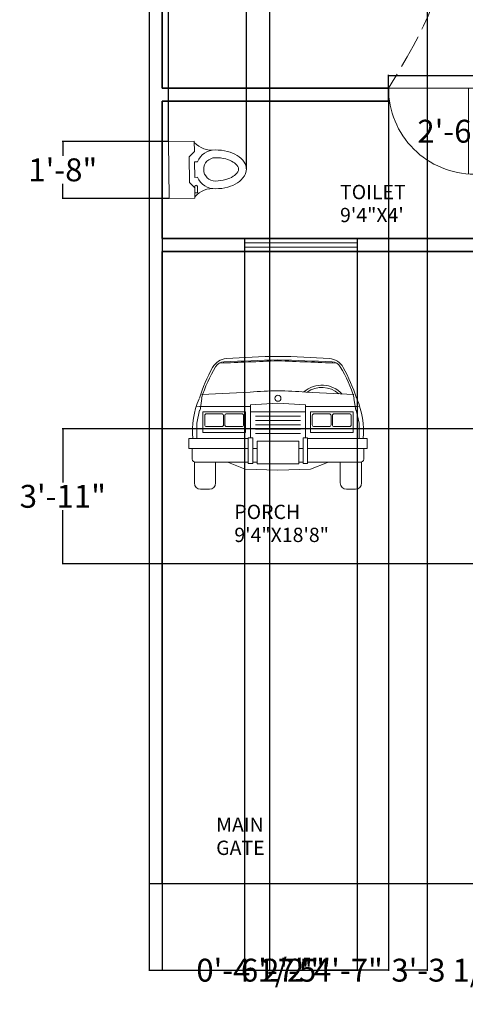
# Model space of a CAD drawing. Units: inches. Extents: x -26 to 385, y 12 to 697.
# Tile 1 of 13: x -20 to 136, y 12 to 356. Entities that reach past the tile are written whole.
import ezdxf

# ---------------------------------------------------------------- set-up
doc = ezdxf.new("R2010")
doc.units = ezdxf.units.IN
doc.header["$MEASUREMENT"] = 0
doc.linetypes.add('ACAD_ISO02W100', pattern=[15, 12, -3])
for name, color, linetype, lineweight in [('A-ANNO-DIMS', 4, 'Continuous', 18), ('A-ANNO-TEXT', 7, 'Continuous', 18), ('A-AREA-IDEN', 4, 'Continuous', 18), ('A-DOOR', 30, 'Continuous', 20), ('A-EQPM-VEHI', 7, 'Continuous', 15), ('A-FLOR-FIXT', 7, 'Continuous', 18), ('A-FLOR-OVHD', 3, 'ACAD_ISO02W100', 13), ('A-GLAZ', 5, 'Continuous', 18), ('A-WALL', 40, 'Continuous', 35), ('C-PROP', 40, 'Continuous', 25)]:
    doc.layers.add(name, color=color, linetype=linetype, lineweight=lineweight)
doc.styles.get("Standard").update_dxf_attribs({"font": 'italic8.shx'})
doc.dimstyles.get("Standard").update_dxf_attribs({"dimtxt": 8, "dimasz": 0.18, "dimexe": 0.18, "dimexo": 0.0625, "dimgap": 0.09, "dimtad": 0, "dimtih": 1, "dimtoh": 1, "dimdec": 4, "dimzin": 0, "dimdsep": 46, "dimlunit": 3, "dimtxsty": 'Standard', "dimcen": 0.09, "dimclrd": 2, "dimclre": 3, "dimclrt": 6, "dimadec": 0, "dimazin": 0, "dimtfac": 1, "dimtdec": 4, "dimtofl": 0, "dimtmove": 0, "dimatfit": 3, "dimfxl": 1, "dimtolj": 1, "dimtzin": 0, "dimarcsym": 0})

# ---------------------------------------------------------------- blocks, each defined once
blk = doc.blocks.new('DOOR-SWING-30IN')
for p, q in [((0, -30), (0, 0)), ((0, 0), (30, 0)), ((0, -2), (30, -2))]:
    blk.add_line(p, q)
blk.add_arc((0, 0), 30, 270, 0)
blk = doc.blocks.new('*D17')
at = {"layer": 'A-ANNO-DIMS', "color": 3, "lineweight": -2, "transparency": 16777216}
for p, q in [((108.79, 332.44), (108.79, 337.06)), ((138.79, 332.44), (138.79, 337.06))]:
    blk.add_line(p, q, dxfattribs=at)
at = {"layer": 'A-ANNO-DIMS', "color": 2, "lineweight": -2, "transparency": 16777216}
for p, q in [((108.97, 336.88), (138.61, 336.88)), ((138.79, 336.88), (138.97, 336.88))]:
    blk.add_line(p, q, dxfattribs=at)
at = {"layer": 'A-ANNO-DIMS', "color": 2, "transparency": 16777216}
for points in [[(108.97, 336.91), (108.97, 336.85), (108.79, 336.88)], [(138.61, 336.91), (138.61, 336.85), (138.79, 336.88)]]:
    blk.add_solid(points, dxfattribs=at)
at = {"layer": 'Defpoints', "color": 0, "transparency": 16777216}
for p in [(138.79, 336.88), (108.79, 332.38), (138.79, 332.38)]:
    blk.add_point(p, dxfattribs=at)
at = {"layer": 'A-ANNO-DIMS', "color": 6, "transparency": 16777216, "insert": (196.21, 336.88), "char_height": 8, "attachment_point": 5}
blk.add_mtext('\\A1;DOOR 2\'-6" TYP.', dxfattribs=at)
blk = doc.blocks.new('*D18')
at = {"layer": 'A-ANNO-DIMS', "color": 3, "lineweight": -2, "transparency": 16777216}
for p, q in [((138.86, 332.38), (143.47, 332.38)), ((138.86, 302.38), (143.47, 302.38))]:
    blk.add_line(p, q, dxfattribs=at)
at = {"layer": 'A-ANNO-DIMS', "color": 2, "lineweight": -2, "transparency": 16777216}
for p, q in [((143.29, 332.2), (143.29, 322.23)), ((143.29, 302.56), (143.29, 312.53))]:
    blk.add_line(p, q, dxfattribs=at)
at = {"layer": 'A-ANNO-DIMS', "color": 2, "transparency": 16777216}
for points in [[(143.26, 332.2), (143.32, 332.2), (143.29, 332.38)], [(143.26, 302.56), (143.32, 302.56), (143.29, 302.38)]]:
    blk.add_solid(points, dxfattribs=at)
at = {"layer": 'Defpoints', "color": 0, "transparency": 16777216}
for p in [(138.79, 332.38), (138.79, 302.38), (143.29, 302.38)]:
    blk.add_point(p, dxfattribs=at)
at = {"layer": 'A-ANNO-DIMS', "color": 6, "transparency": 16777216, "insert": (143.29, 317.38), "char_height": 8, "attachment_point": 5}
blk.add_mtext('\\A1;2\'-6" TYP.', dxfattribs=at)
blk = doc.blocks.new('*D29')
at = {"layer": 'A-ANNO-DIMS', "color": 3, "lineweight": -2, "transparency": 16777216}
for p, q in [((67.17, 549.17), (67.17, 23.95)), ((122.29, 549.17), (122.29, 23.95))]:
    blk.add_line(p, q, dxfattribs=at)
at = {"layer": 'A-ANNO-DIMS', "color": 2, "lineweight": -2, "transparency": 16777216}
for p, q in [((67.35, 24.13), (76.92, 24.13)), ((122.11, 24.13), (112.53, 24.13))]:
    blk.add_line(p, q, dxfattribs=at)
at = {"layer": 'A-ANNO-DIMS', "color": 2, "transparency": 16777216}
for points in [[(67.35, 24.16), (67.35, 24.1), (67.17, 24.13)], [(122.11, 24.16), (122.11, 24.1), (122.29, 24.13)]]:
    blk.add_solid(points, dxfattribs=at)
at = {"layer": 'Defpoints', "color": 0, "transparency": 16777216}
for p in [(67.17, 549.23), (122.29, 549.23), (122.29, 24.13)]:
    blk.add_point(p, dxfattribs=at)
at = {"layer": 'A-ANNO-DIMS', "color": 6, "transparency": 16777216, "insert": (94.73, 24.13), "char_height": 8, "attachment_point": 5}
blk.add_mtext('\\A1;4\'-7"', dxfattribs=at)
blk = doc.blocks.new('*D32')
at = {"layer": 'A-ANNO-DIMS', "color": 3, "lineweight": -2, "transparency": 16777216}
for p, q in [((239.83, 213.39), (-5.3, 213.39)), ((239.83, 166.14), (-5.3, 166.14))]:
    blk.add_line(p, q, dxfattribs=at)
at = {"layer": 'A-ANNO-DIMS', "color": 2, "lineweight": -2, "transparency": 16777216}
for p, q in [((-5.12, 213.21), (-5.12, 194.62)), ((-5.12, 166.32), (-5.12, 184.91))]:
    blk.add_line(p, q, dxfattribs=at)
at = {"layer": 'A-ANNO-DIMS', "color": 2, "transparency": 16777216}
for points in [[(-5.15, 213.21), (-5.09, 213.21), (-5.12, 213.39)], [(-5.15, 166.32), (-5.09, 166.32), (-5.12, 166.14)]]:
    blk.add_solid(points, dxfattribs=at)
at = {"layer": 'Defpoints', "color": 0, "transparency": 16777216}
for p in [(-5.12, 213.39), (239.89, 213.39), (239.89, 166.14)]:
    blk.add_point(p, dxfattribs=at)
at = {"layer": 'A-ANNO-DIMS', "color": 6, "transparency": 16777216, "insert": (-5.12, 189.76), "char_height": 8, "attachment_point": 5}
blk.add_mtext('\\A1;3\'-11"', dxfattribs=at)
blk = doc.blocks.new('*D33')
at = {"layer": 'A-ANNO-DIMS', "color": 3, "lineweight": -2, "transparency": 16777216}
for p, q in [((58.47, 279.82), (58.47, 23.95)), ((97.85, 279.82), (97.85, 23.95))]:
    blk.add_line(p, q, dxfattribs=at)
at = {"layer": 'A-ANNO-DIMS', "color": 2, "lineweight": -2, "transparency": 16777216}
for p, q in [((58.65, 24.13), (97.67, 24.13)), ((97.85, 24.13), (98.03, 24.13))]:
    blk.add_line(p, q, dxfattribs=at)
at = {"layer": 'A-ANNO-DIMS', "color": 2, "transparency": 16777216}
for points in [[(58.65, 24.16), (58.65, 24.1), (58.47, 24.13)], [(97.67, 24.16), (97.67, 24.1), (97.85, 24.13)]]:
    blk.add_solid(points, dxfattribs=at)
at = {"layer": 'Defpoints', "color": 0, "transparency": 16777216}
for p in [(58.47, 279.88), (97.85, 279.88), (97.85, 24.13)]:
    blk.add_point(p, dxfattribs=at)
at = {"layer": 'A-ANNO-DIMS', "color": 6, "transparency": 16777216, "insert": (131.26, 24.13), "char_height": 8, "attachment_point": 5}
blk.add_mtext('\\A1;3\'-3 1/2"', dxfattribs=at)
blk = doc.blocks.new('*D34')
at = {"layer": 'A-ANNO-DIMS', "color": 3, "lineweight": -2, "transparency": 16777216}
for p, q in [((29.63, 279.82), (29.63, 23.95)), ((58.47, 279.82), (58.47, 23.95))]:
    blk.add_line(p, q, dxfattribs=at)
at = {"layer": 'A-ANNO-DIMS', "color": 2, "lineweight": -2, "transparency": 16777216}
for p, q in [((29.81, 24.13), (58.29, 24.13)), ((58.47, 24.13), (58.65, 24.13))]:
    blk.add_line(p, q, dxfattribs=at)
at = {"layer": 'A-ANNO-DIMS', "color": 2, "transparency": 16777216}
for points in [[(29.81, 24.16), (29.81, 24.1), (29.63, 24.13)], [(58.29, 24.16), (58.29, 24.1), (58.47, 24.13)]]:
    blk.add_solid(points, dxfattribs=at)
at = {"layer": 'Defpoints', "color": 0, "transparency": 16777216}
for p in [(29.63, 279.88), (58.47, 279.88), (58.47, 24.13)]:
    blk.add_point(p, dxfattribs=at)
at = {"layer": 'A-ANNO-DIMS', "color": 6, "transparency": 16777216, "insert": (76.64, 24.13), "char_height": 8, "attachment_point": 5}
blk.add_mtext('\\A1;2\'-5"', dxfattribs=at)
blk = doc.blocks.new('*D40')
at = {"layer": 'A-ANNO-DIMS', "color": 3, "lineweight": -2, "transparency": 16777216}
for p, q in [((31.75, 313.84), (-5.3, 313.84)), ((31.96, 293.92), (-5.3, 293.92))]:
    blk.add_line(p, q, dxfattribs=at)
at = {"layer": 'A-ANNO-DIMS', "color": 2, "lineweight": -2, "transparency": 16777216}
for p, q in [((-5.12, 313.66), (-5.12, 308.73)), ((-5.12, 294.1), (-5.12, 299.03))]:
    blk.add_line(p, q, dxfattribs=at)
at = {"layer": 'A-ANNO-DIMS', "color": 2, "transparency": 16777216}
for points in [[(-5.15, 313.66), (-5.09, 313.66), (-5.12, 313.84)], [(-5.15, 294.1), (-5.09, 294.1), (-5.12, 293.92)]]:
    blk.add_solid(points, dxfattribs=at)
at = {"layer": 'Defpoints', "color": 0, "transparency": 16777216}
for p in [(31.81, 313.84), (-5.12, 293.92), (32.02, 293.92)]:
    blk.add_point(p, dxfattribs=at)
at = {"layer": 'A-ANNO-DIMS', "color": 6, "transparency": 16777216, "insert": (-5.12, 303.88), "char_height": 8, "attachment_point": 5}
blk.add_mtext('\\A1;1\'-8"', dxfattribs=at)
blk = doc.blocks.new('*D41')
at = {"layer": 'A-ANNO-DIMS', "color": 3, "lineweight": -2, "transparency": 16777216}
for p, q in [((31.81, 313.9), (31.81, 684.81)), ((59.08, 304.23), (59.08, 684.81))]:
    blk.add_line(p, q, dxfattribs=at)
at = {"layer": 'A-ANNO-DIMS', "color": 2, "lineweight": -2, "transparency": 16777216}
for p, q in [((31.99, 684.63), (58.9, 684.63)), ((59.08, 684.63), (59.26, 684.63))]:
    blk.add_line(p, q, dxfattribs=at)
at = {"layer": 'A-ANNO-DIMS', "color": 2, "transparency": 16777216}
for points in [[(31.99, 684.66), (31.99, 684.6), (31.81, 684.63)], [(58.9, 684.66), (58.9, 684.6), (59.08, 684.63)]]:
    blk.add_solid(points, dxfattribs=at)
at = {"layer": 'Defpoints', "color": 0, "transparency": 16777216}
for p in [(59.08, 684.63), (31.81, 313.84), (59.08, 304.16)]:
    blk.add_point(p, dxfattribs=at)
at = {"layer": 'A-ANNO-DIMS', "color": 6, "transparency": 16777216, "insert": (92.49, 684.63), "char_height": 8, "attachment_point": 5}
blk.add_mtext('\\A1;2\'-3 1/2"', dxfattribs=at)
blk = doc.blocks.new('*D43')
at = {"layer": 'A-ANNO-DIMS', "color": 3, "lineweight": -2, "transparency": 16777216}
for p, q in [((25.13, 54.32), (25.13, 23.95)), ((29.63, 54.32), (29.63, 23.95))]:
    blk.add_line(p, q, dxfattribs=at)
at = {"layer": 'A-ANNO-DIMS', "color": 2, "lineweight": -2, "transparency": 16777216}
for p, q in [((25.31, 24.13), (29.45, 24.13)), ((29.63, 24.13), (29.81, 24.13))]:
    blk.add_line(p, q, dxfattribs=at)
at = {"layer": 'A-ANNO-DIMS', "color": 2, "transparency": 16777216}
for points in [[(25.31, 24.16), (25.31, 24.1), (25.13, 24.13)], [(29.45, 24.16), (29.45, 24.1), (29.63, 24.13)]]:
    blk.add_solid(points, dxfattribs=at)
at = {"layer": 'Defpoints', "color": 0, "transparency": 16777216}
for p in [(25.13, 54.38), (29.63, 54.38), (29.63, 24.13)]:
    blk.add_point(p, dxfattribs=at)
at = {"layer": 'A-ANNO-DIMS', "color": 6, "transparency": 16777216, "insert": (63.04, 24.13), "char_height": 8, "attachment_point": 5}
blk.add_mtext('\\A1;0\'-4 1/2"', dxfattribs=at)
blk = doc.blocks.new('*D47')
at = {"layer": 'A-ANNO-DIMS', "color": 3, "lineweight": -2, "transparency": 16777216}
for p, q in [((29.63, 327.82), (29.63, 23.95)), ((108.79, 327.82), (108.79, 23.95))]:
    blk.add_line(p, q, dxfattribs=at)
at = {"layer": 'A-ANNO-DIMS', "color": 2, "lineweight": -2, "transparency": 16777216}
for p, q in [((29.81, 24.13), (51.41, 24.13)), ((108.61, 24.13), (87.02, 24.13))]:
    blk.add_line(p, q, dxfattribs=at)
at = {"layer": 'A-ANNO-DIMS', "color": 2, "transparency": 16777216}
for points in [[(29.81, 24.16), (29.81, 24.1), (29.63, 24.13)], [(108.61, 24.16), (108.61, 24.1), (108.79, 24.13)]]:
    blk.add_solid(points, dxfattribs=at)
at = {"layer": 'Defpoints', "color": 0, "transparency": 16777216}
for p in [(29.63, 327.88), (108.79, 327.88), (108.79, 24.13)]:
    blk.add_point(p, dxfattribs=at)
at = {"layer": 'A-ANNO-DIMS', "color": 6, "transparency": 16777216, "insert": (69.21, 24.13), "char_height": 8, "attachment_point": 5}
blk.add_mtext('\\A1;6\'-7"', dxfattribs=at)

msp = doc.modelspace()

# ---------------------------------------------------------------- linework, layer by layer
at = {"layer": 'A-EQPM-VEHI'}
for p, q in [((43.52309, 223.97111), (42.85778, 219.9024)), ((60.39116, 226.18572), (43.52309, 225.29953)), ((79.84318, 226.18572), (96.71125, 225.29953)), ((96.71125, 223.97111), (97.37656, 219.9024)), ((43.01615, 221.16936), (41.74919, 221.32773)), ((42.70356, 221.18633), (60.51804, 221.18633)), ((60.51804, 221.74383), (70.11717, 222.33442)), ((60.51804, 210.2496), (60.51804, 221.74383)), ((79.7163, 221.74383), (70.11717, 222.33442)), ((79.7163, 210.2496), (79.7163, 221.74383)), ((97.53078, 221.18633), (79.7163, 221.18633)), ((97.21819, 221.16936), (98.48515, 221.32773)), ((42.71571, 219.85792), (41.74919, 215.30968)), ((43.83595, 212.09194), (43.83595, 219.28259)), ((43.83595, 219.28259), (58.7398, 219.28259)), ((44.49774, 217.94019), (44.49774, 214.79154)), ((50.4349, 218.59311), (45.15065, 218.59311)), ((51.08782, 217.94019), (51.08782, 214.79154)), ((51.53662, 217.94019), (51.53662, 214.79154)), ((57.47378, 218.59311), (52.18953, 218.59311)), ((58.12669, 214.79154), (58.12669, 217.94019)), ((58.7398, 219.28259), (58.7398, 212.09194)), ((60.51804, 219.28259), (79.7163, 219.28259)), ((78.01892, 217.75578), (62.21542, 217.75578)), ((96.39839, 219.28259), (81.49454, 219.28259)), ((81.49454, 219.28259), (81.49454, 212.09194)), ((82.10765, 214.79154), (82.10765, 217.94019)), ((82.76056, 218.59311), (88.04481, 218.59311)), ((88.69772, 217.94019), (88.69772, 214.79154)), ((89.14652, 217.94019), (89.14652, 214.79154)), ((89.79944, 218.59311), (95.08369, 218.59311)), ((95.7366, 217.94019), (95.7366, 214.79154)), ((96.39839, 212.09194), (96.39839, 219.28259)), ((97.51863, 219.85792), (98.48515, 215.30968)), ((41.74919, 215.30968), (41.74919, 209.94942)), ((45.15065, 214.13863), (50.4349, 214.13863)), ((52.18953, 214.13863), (57.47378, 214.13863)), ((78.01892, 216.25078), (62.21542, 216.25078)), ((78.01892, 214.74578), (62.21542, 214.74578)), ((88.04481, 214.13863), (82.76056, 214.13863)), ((95.08369, 214.13863), (89.79944, 214.13863)), ((98.48515, 215.30968), (98.48515, 209.94942)), ((38.90862, 209.94942), (59.74715, 209.94942)), ((38.90862, 206.4827), (38.90862, 209.94942)), ((58.7398, 212.09194), (43.83595, 212.09194)), ((59.74715, 210.2496), (59.74715, 201.2559)), ((61.28893, 210.2496), (59.74715, 210.2496)), ((61.28893, 201.2559), (61.28893, 210.2496)), ((78.01892, 213.24078), (62.21542, 213.24078)), ((78.01892, 211.73577), (62.21542, 211.73577)), ((78.94541, 210.2496), (80.48719, 210.2496)), ((78.94541, 201.2559), (78.94541, 210.2496)), ((80.48719, 210.2496), (80.48719, 201.2559)), ((101.32572, 209.94942), (80.48719, 209.94942)), ((81.49454, 212.09194), (96.39839, 212.09194)), ((101.32572, 206.4827), (101.32572, 209.94942)), ((62.8307, 201.17364), (62.8307, 209.05709)), ((62.8307, 209.05709), (77.40364, 209.05709)), ((77.40364, 201.17364), (77.40364, 209.05709)), ((38.90862, 206.4827), (59.74715, 206.4827)), ((40.07105, 202.71282), (40.07105, 206.49837)), ((61.28893, 206.4827), (62.8307, 206.4827)), ((77.40364, 206.4827), (78.94541, 206.4827)), ((101.32572, 206.4827), (80.48719, 206.4827)), ((100.16329, 202.71282), (100.16329, 206.49837)), ((40.87494, 194.43858), (40.87494, 201.68757)), ((41.17393, 201.68757), (59.74715, 201.68757)), ((48.32687, 201.68757), (48.32687, 194.43858)), ((58.68103, 199.27878), (52.7722, 201.6394)), ((59.74715, 201.2559), (61.28893, 201.2559)), ((61.28893, 201.68757), (62.8307, 201.68757)), ((77.40364, 201.17364), (62.8307, 201.17364)), ((78.94541, 201.68757), (77.40364, 201.68757)), ((80.48719, 201.2559), (78.94541, 201.2559)), ((99.06041, 201.68757), (80.48719, 201.68757)), ((81.55331, 199.27878), (87.46214, 201.6394)), ((91.90747, 201.68757), (91.90747, 194.43858)), ((99.3594, 194.43858), (99.3594, 201.68757)), ((58.68103, 199.27878), (70.11717, 198.88443)), ((81.55331, 199.27878), (70.11717, 198.88443)), ((46.15049, 192.26219), (43.05132, 192.26219)), ((94.08385, 192.26219), (97.18302, 192.26219))]:
    msp.add_line(p, q, dxfattribs=at)
msp.add_circle((70.11717, 224.03012), 1.04972, dxfattribs=at)
for centre, radius, start, end in [((52.56766, 231.80627), 6.09387, 94.3522531, 150.4523105), ((-649.67099, 18854.07108), 18630.4755, 272.155969962, 272.214172709), ((72.72883, -23.40829), 262.11246, 90.570898, 94.5129852), ((67.50551, -23.40829), 262.11246, 85.4870148, 89.429102), ((789.90533, 18854.07108), 18630.4755, 267.785827291, 267.844030038), ((87.66668, 231.80627), 6.09387, 29.5476895, 85.6477469), ((101.7158, 205.06552), 62.05167, 151.3520748, 162.1730481), ((92.5461, 208.75684), 51.47934, 149.2485315, 162.6299285), ((51.33669, 233.30406), 3.48221, 92.1583471, 149.6553306), ((-649.67099, 18853.68338), 18630.4755, 272.151105889, 272.214172709), ((789.90533, 18853.68338), 18630.4755, 267.785827291, 267.848894111), ((88.89765, 233.30406), 3.48221, 30.3446694, 87.8416529), ((47.68824, 208.75684), 51.47934, 17.3700715, 30.7514685), ((38.51854, 205.06552), 62.05167, 17.8269519, 28.6479252), ((85.51357, 219.02994), 9.59405, 42.5392666, 131.3169517), ((85.51357, 219.02994), 8.79496, 48.1321669, 125.8531041), ((68.6573, 212.57431), 28.45106, 156.6261933, 185.2936243), ((72.72883, 66.85513), 159.80755, 90.9363992, 94.4278296), ((67.50551, 66.85513), 159.80755, 85.5721704, 89.0636008), ((71.57704, 212.57431), 28.45106, 354.7063757, 23.3738067), ((45.15065, 217.94019), 0.65291, 90, 180), ((50.4349, 217.94019), 0.65291, 0, 90), ((52.18953, 217.94019), 0.65291, 90, 180), ((57.47378, 217.94019), 0.65291, 0, 90), ((82.76056, 217.94019), 0.65291, 90, 180), ((88.04481, 217.94019), 0.65291, 0, 90), ((89.79944, 217.94019), 0.65291, 90, 180), ((95.08369, 217.94019), 0.65291, 0, 90), ((45.15065, 214.79154), 0.65291, 180, 270), ((50.4349, 214.79154), 0.65291, 270, 0), ((52.18953, 214.79154), 0.65291, 180, 270), ((57.47378, 214.79154), 0.65291, 270, 0), ((82.76056, 214.79154), 0.65291, 180, 270), ((88.04481, 214.79154), 0.65291, 270, 0), ((89.79944, 214.79154), 0.65291, 180, 270), ((95.08369, 214.79154), 0.65291, 270, 0), ((41.34638, 202.9934), 1.30583, 192.4074185, 270), ((98.88796, 202.9934), 1.30583, 270, 347.5925815), ((43.05132, 194.43858), 2.17638, 180, 270), ((46.15049, 194.43858), 2.17638, 270, 0), ((94.08385, 194.43858), 2.17638, 180, 270), ((97.18302, 194.43858), 2.17638, 270, 0)]:
    msp.add_arc(centre, radius, start, end, dxfattribs=at)
at = {"layer": 'A-FLOR-FIXT'}
for p, q in [((31.81206, 313.83916), (40.86667, 313.9337)), ((32.02006, 293.91902), (31.81206, 313.83916)), ((40.86667, 313.9337), (40.90448, 310.31186)), ((39.11247, 308.48203), (40.90448, 310.31186)), ((39.20702, 299.42742), (39.11247, 308.48203)), ((40.9423, 306.69002), (41.96197, 306.70066)), ((40.9423, 306.69002), (40.99903, 301.25725)), ((39.20702, 299.42742), (41.03685, 297.63541)), ((40.99903, 301.25725), (42.0187, 301.2679)), ((41.07466, 294.01357), (41.03212, 298.08814)), ((41.96122, 295.83394), (41.93758, 298.09759)), ((32.02006, 293.91902), (41.07466, 294.01357)), ((41.05576, 295.82449), (41.96122, 295.83394))]:
    msp.add_line(p, q, dxfattribs=at)
for centre, radius, start, end in [((46.95399, 318.89794), 8.14503, 221.6872316, 278.3971556), ((48.21435, 304.04927), 6.79132, 90.5982386, 157.0200606), ((48.32433, 293.51492), 17.32625, 76.0839883, 90.5982004), ((49.61505, 298.72423), 11.95942, 58.5928455, 76.0839809), ((48.21435, 304.04927), 4.07479, 90.5982386, 270.5982386), ((48.32434, 293.51493), 14.60971, 76.0839959, 90.5982081), ((49.61505, 298.72423), 9.24289, 58.5928422, 76.0839775), ((51.6305, 302.02514), 5.37532, 34.1323677, 58.5928282), ((51.6305, 302.02514), 8.09186, 34.1323633, 58.5928239), ((54.71663, 304.11716), 4.36348, 0.5982853, 34.1323064), ((51.58749, 306.14428), 5.37532, 302.603649, 327.0641096), ((54.71664, 304.11716), 1.64695, 0.5982597, 34.1322807), ((54.71664, 304.11716), 1.64695, 327.0641965, 0.5982175), ((54.71663, 304.11717), 4.36348, 327.0641709, 0.5981919), ((48.21435, 304.04927), 6.79132, 204.1764166, 270.5982386), ((48.10435, 314.58361), 14.60971, 270.5982692, 285.1124813), ((49.50355, 309.4024), 9.24289, 285.1124997, 302.6036351), ((51.58749, 306.14429), 8.09186, 302.6036534, 327.0641139), ((41.48485, 298.09287), 0.45276, 0.5982386, 180.5982386), ((47.26432, 289.17752), 8.14503, 82.7993216, 139.5092456), ((48.10434, 314.58362), 17.32625, 270.5982768, 285.1124889), ((49.50356, 309.40239), 11.95942, 285.1124964, 302.6036318)]:
    msp.add_arc(centre, radius, start, end, dxfattribs=at)
at = {"layer": 'A-FLOR-OVHD'}
msp.add_open_spline([(126.19858, 477.37909), (100.28194, 454.00117), (57.72956, 415.61709), (142.76157, 388.96462), (120.64168, 352.11697), (108.79289, 332.37909)], degree=3, knots=[0, 0, 0, 0, 74.502604677, 122.325399102, 177.493963659, 177.493963659, 177.493963659, 177.493963659], dxfattribs=at)
at = {"layer": 'A-GLAZ'}
for p, q in [((58.46784, 279.87909), (58.46784, 275.37909)), ((97.84659, 279.87909), (58.46784, 279.87909)), ((97.84659, 275.37909), (97.84659, 279.87909)), ((58.46784, 278.37909), (97.84659, 278.37909)), ((58.46784, 276.87909), (97.84659, 276.87909)), ((58.46784, 275.37909), (97.84659, 275.37909))]:
    msp.add_line(p, q, dxfattribs=at)
at = {"layer": 'A-WALL'}
for p, q in [((29.62932, 477.37909), (29.62932, 332.37909)), ((108.79289, 332.37909), (29.62932, 332.37909)), ((108.79289, 332.37909), (108.79289, 327.87909)), ((29.62932, 327.87909), (29.62932, 279.87909)), ((108.79289, 327.87909), (29.62932, 327.87909)), ((141.62932, 279.87909), (29.62932, 279.87909)), ((29.62932, 275.37909), (29.62932, 54.37909)), ((141.62932, 275.37909), (29.62932, 275.37909))]:
    msp.add_line(p, q, dxfattribs=at)
at = {"layer": 'C-PROP'}
for p, q in [((25.12932, 654.37909), (25.12932, 54.37909)), ((25.12932, 54.37909), (325.12932, 54.37909))]:
    msp.add_line(p, q, dxfattribs=at)

# ---------------------------------------------------------------- block references
at = {"layer": 'A-DOOR', "rotation": 269.9999999999999}
msp.add_blockref('DOOR-SWING-30IN', (138.79289, 332.37909), dxfattribs=at)

# ---------------------------------------------------------------- texts
at = {"layer": 'A-ANNO-TEXT'}
for s, p in [('MAIN', (48.50875, 72.49598)), ('GATE', (48.50875, 64.40075))]:
    msp.add_text(s, height=5, dxfattribs=at).set_placement(p)
at = {"layer": 'A-AREA-IDEN'}
for s, p in [('TOILET', (91.82988, 293.63297)), ('9\'4"X4\'', (91.82988, 285.60091)), ('PORCH', (54.85639, 181.82022)), ('9\'4"X18\'8"', (54.85639, 173.78816))]:
    msp.add_text(s, height=5, dxfattribs=at).set_placement(p)

# ---------------------------------------------------------------- dimensions: what is measured, and where the dimension line sits
at = {"layer": 'A-ANNO-DIMS'}
for base, p1, p2, picture, middle in [((59.07988, 684.62909), (31.81206, 313.83916), (59.07988, 304.16272), '*D41', (92.49274, 684.62909)), ((122.28508, 24.12909), (67.16708, 549.23099), (122.28508, 549.23099), '*D29', (94.72608, 24.12909)), ((108.79289, 24.12909), (29.62932, 327.87909), (108.79289, 327.87909), '*D47', (69.21111, 24.12909)), ((58.46784, 24.12909), (29.62932, 279.87909), (58.46784, 279.87909), '*D34', (76.6426, 24.12909)), ((97.84659, 24.12909), (58.46784, 279.87909), (97.84659, 279.87909), '*D33', (131.25945, 24.12909)), ((29.62932, 24.12909), (25.12932, 54.37909), (29.62932, 54.37909), '*D43', (63.04218, 24.12909))]:
    dim = msp.add_linear_dim(base=base, p1=p1, p2=p2, dimstyle='Standard', override={"dimdec": 1, "dimlfac": 1, "dimrnd": 0, "dimzin": 1, "dimdsep": 46, "dimlunit": 4, "dimfrac": 2}, dxfattribs=at)
    dim.commit()
    dim.dimension.update_dxf_attribs({"geometry": picture, "text_midpoint": middle})
dim = msp.add_linear_dim(base=(138.79289, 336.87909), p1=(108.79289, 332.37909), p2=(138.79289, 332.37909), text='DOOR <> TYP.', dimstyle='Standard', override={"dimdec": 1, "dimlfac": 1, "dimrnd": 0, "dimzin": 1, "dimdsep": 46, "dimlunit": 4, "dimfrac": 2}, dxfattribs=at)
dim.commit()
dim.dimension.update_dxf_attribs({"geometry": '*D17', "text_midpoint": (196.20575, 336.87909)})
dim = msp.add_linear_dim(base=(143.29289, 302.37909), p1=(138.79289, 332.37909), p2=(138.79289, 302.37909), angle=270, text='<> TYP.', dimstyle='Standard', override={"dimdec": 1, "dimlfac": 1, "dimrnd": 0, "dimzin": 1, "dimdsep": 46, "dimlunit": 4, "dimfrac": 2}, dxfattribs=at)
dim.commit()
dim.dimension.update_dxf_attribs({"geometry": '*D18', "text_midpoint": (143.29289, 317.37909)})
for base, p1, p2, picture, middle in [((-5.12068, 293.91902), (31.81206, 313.83916), (32.02006, 293.91902), '*D40', (-5.12068, 303.87909)), ((-5.12068, 213.38513), (239.88756, 166.14113), (239.88756, 213.38513), '*D32', (-5.12068, 189.76313))]:
    dim = msp.add_linear_dim(base=base, p1=p1, p2=p2, angle=90, dimstyle='Standard', override={"dimdec": 1, "dimlfac": 1, "dimrnd": 0, "dimzin": 1, "dimdsep": 46, "dimlunit": 4, "dimfrac": 2}, dxfattribs=at)
    dim.commit()
    dim.dimension.update_dxf_attribs({"geometry": picture, "text_midpoint": middle})

doc.saveas('drawing.dxf')
